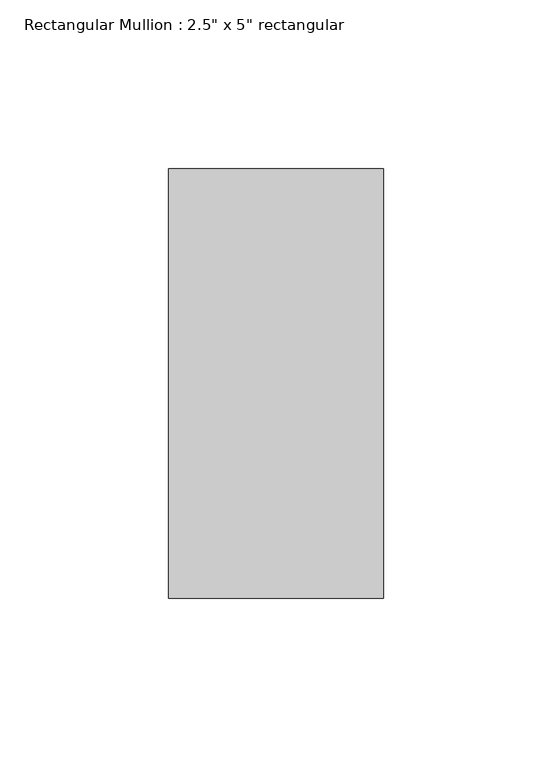
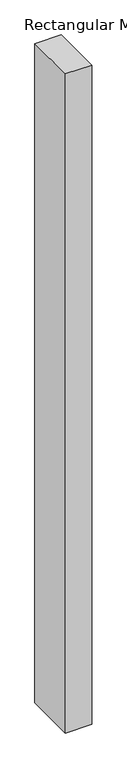
"""IFC4 building model written with IfcOpenShell, lengths in millimetres: member geometry."""

from ifc_helpers import new_model, si_unit, frame, origin, place, context, project, spatial, polyline, outline, extrude, source, transform, mapped, element, save


def member_443975aa(model_context):
    return source(origin(), model_context, "Body", "SweptSolid", [
        extrude(outline(polyline([(0.0, 63.5), (0.0, -63.5), (-63.5, -63.5), (-63.5, 63.5), (0.0, 63.5)])), frame((0.0, 0.0, -1677.4900448), z_axis=(0.0, 0.0, 1.0), x_axis=(1.0, 0.0, 0.0)), (0.0, 0.0, 1.0), 1677.4900448),
    ])


if __name__ == "__main__":
    model = new_model("IFC4")
    model_context = context("Model", 3, world=origin())
    ifc_project = project(units=[si_unit("LENGTHUNIT", "METRE", prefix="MILLI")], contexts=[model_context])
    site = spatial("IfcSite", under=ifc_project)
    building = spatial("IfcBuilding", under=site)
    placement = place(None, origin())
    member_shape = member_443975aa(model_context)
    element("IfcMember", 1, ObjectType="Rectangular Mullion : 2.5\" x 5\" rectangular", at=placement, inside=building, context=model_context, shape_type="MappedRepresentation", body=[
        mapped(member_shape, transform((0.0, 0.0, 0.0), x_axis=(1.0, 0.0, 0.0), y_axis=(0.0, 1.0, 0.0), z_axis=(0.0, 0.0, 1.0))),
    ])
    save(model, "model.ifc")

# Revit data of these elements
# Type "Rectangular Mullion : 2.5\" x 5\" rectangular"
#   built-in parameter 1007304 = 0.416667 (stored number, unit not read)
#   built-in parameter 1007301 = 0.104167 (stored number, unit not read)
#   built-in parameter 1007300 = 0.104167 (stored number, unit not read)
# Element 1 (IfcMember, "Rectangular Mullion : 2.5\" x 5\" rectangular")
#   Materials on its faces: "Aluminum"
# Materials
#   "Aluminum": class "Metal", colour RGB 247 247 247, transparency 0, Description = "Aluminum 6061", Cost = 0
